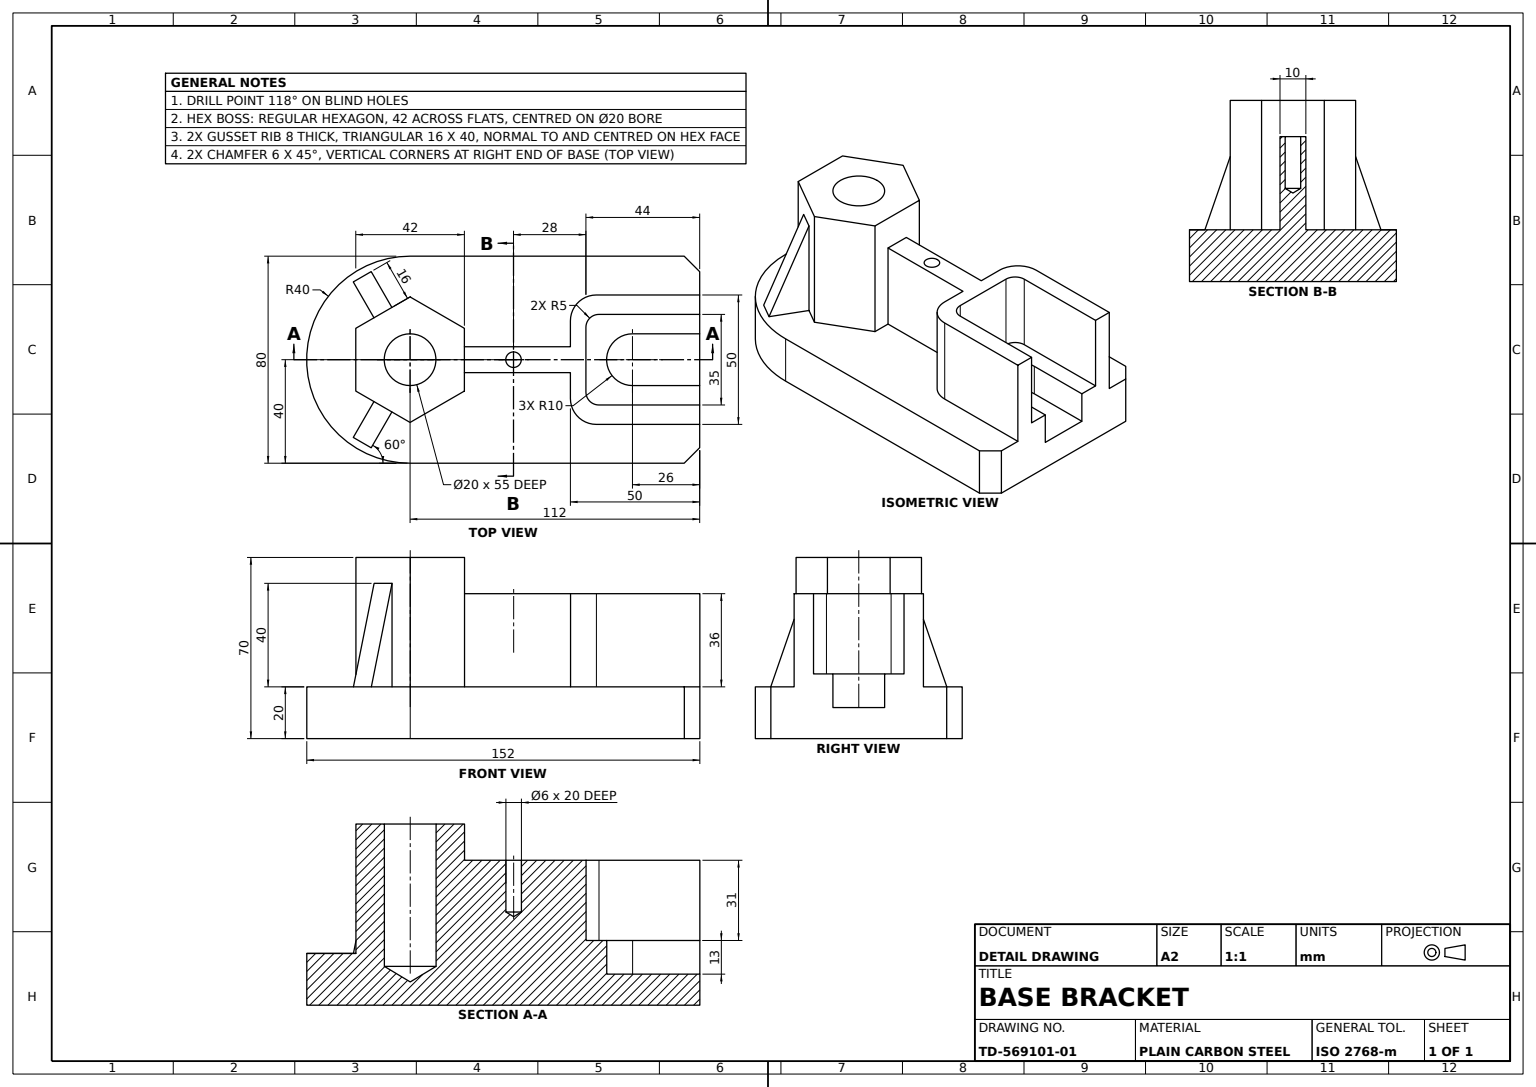
SolidWorks part; units mm, degrees
material "Plain Carbon Steel"
ref_plane "Front Plane" through (0, 0, 0) normal (0, 0, 1) x (1, 0, 0)
ref_plane "Top Plane" through (0, 0, 0) normal (0, 1, 0) x (1, 0, 0)
ref_plane "Right Plane" through (0, 0, 0) normal (1, 0, 0) x (0, 0, -1)
sketch "Base Plate Sketch" plane through (0, 0, 0) normal (0, 1, 0) x (1, 0, 0)
  line L0 (0, 40) -> (106, 40)
  line L1 (112, 34) -> (112, -34)
  line L2 (106, -40) -> (0, -40)
  line L3 (106, 40) -> (112, 34)
  line L4 (112, -34) -> (106, -40)
  arc A0 (0, 40) -> (0, -40) centre (0, 0) ccw
  point P4 (112, 40)
  point P5 (112, -40)
  dimension "D1" = 80
  dimension "D2" = 112
  dimension "D3" = 6
  dimension "D4" = 45
  dimension "D5" = 6
  dimension "D6" = 45
extrude "Base Plate" add sketch "Base Plate Sketch" along normal blind 20
sketch "Hex Boss Sketch" plane through (0, 20, 0) normal (0, 1, 0) x (1, 0, 0)
  line L1 (0, 24.2487) -> (-21, 12.1244)
  line L2 (-21, 12.1244) -> (-21, -12.1244)
  line L3 (-21, -12.1244) -> (0, -24.2487)
  line L4 (0, -24.2487) -> (21, -12.1244)
  line L5 (21, -12.1244) -> (21, 12.1244)
  line L6 (21, 12.1244) -> (0, 24.2487)
  circle A0 centre (0, 0) radius 21 construction
  dimension "D1" = 42
extrude "Hex Mounting Boss" add sketch "Hex Boss Sketch" along normal blind 50
sketch "Gusset Rib 1 Sketch" plane through (-10.5, 0, 18.1865) normal (-0.5, 0, 0.866) x (0.866, 0, 0.5)
  line L0 (-12.1244, 20) -> (12.1244, 20) construction
  line L1 (-4, 60) -> (4, 60)
  line L2 (-4, 60) -> (-4, 20)
  line L3 (-4, 20) -> (4, 20)
  line L4 (4, 60) -> (4, 20)
  line L5 (-12.1244, 70) -> (12.1244, 70) construction
  point P8 (0, 70)
  dimension "D1" = 4
  dimension "D2" = 8
  dimension "D3" = 40
extrude "Gusset Rib 1" add sketch "Gusset Rib 1 Sketch" along normal blind 16
sketch "Rib 1 Trim Sketch" plane through (3.4641, 0, 2) normal (0.866, 0, 0.5) x (0.5, 0, -0.866)
  line L0 (-21, 60) -> (-37, 20)
  line L1 (-21, 60) -> (-37, 60)
  line L2 (-37, 60) -> (-37, 20)
extrude "Rib 1 Trim Cut" cut sketch "Rib 1 Trim Sketch" against normal blind 16
sketch "Gusset Rib 2 Sketch" plane through (-10.5, 0, -18.1865) normal (-0.5, 0, -0.866) x (-0.866, 0, 0.5)
  line L0 (-12.1244, 20) -> (12.1244, 20) construction
  line L1 (-4, 60) -> (4, 60)
  line L2 (-4, 60) -> (-4, 20)
  line L3 (-4, 20) -> (4, 20)
  line L4 (4, 60) -> (4, 20)
  line L5 (-12.1244, 70) -> (12.1244, 70) construction
  point P8 (0, 70)
  dimension "D1" = 4
  dimension "D2" = 8
  dimension "D3" = 40
extrude "Gusset Rib 2" add sketch "Gusset Rib 2 Sketch" along normal blind 16
sketch "Rib 2 Trim Sketch" plane through (-3.4641, 0, 2) normal (-0.866, 0, 0.5) x (0.5, 0, 0.866)
  line L0 (-21, 60) -> (-37, 20)
  line L1 (-37, 20) -> (-37, 60)
  line L2 (-37, 60) -> (-21, 60)
extrude "Rib 2 Trim Cut" cut sketch "Rib 2 Trim Sketch" against normal blind 16
hole_wizard "Boss Bore Ø20" positions "Sketch16" profile "Sketch17" hole size "Ø20.0" standard "ISO"
sketch "Sketch16" plane through (0, 70, 0) normal (0, 1, 0) x (1, 0, 0)
  point P0 (0, 0)
sketch "Sketch17" plane through (0, 70, 0) normal (1, 0, 0) x (0, 0, 1)
  line L0 (0, 0) -> (0, 61.0086)
  line L1 (0, 61.0086) -> (10, 55)
  line L2 (10, 55) -> (10, 0)
  line L5 (10, 0) -> (0, 0)
  line L10 (0, 61.0086) -> (-10, 55) construction
  line L11 (0, -6.35) -> (0, 107.95) construction
  dimension "Hole Dia." = 20
  dimension "Hole Depth" = 55
  dimension "Drill Angle" = 118
sketch "Shaft Housing Sketch" plane through (0, 20, 0) normal (0, 1, 0) x (1, 0, 0)
  line L0 (112, -34) -> (112, 34) construction
  line L1 (112, 25) -> (62, 25)
  line L2 (112, 25) -> (112, -25)
  line L3 (112, -25) -> (62, -25)
  line L4 (62, 25) -> (62, 5)
  line L5 (21, -12.1244) -> (21, 12.1244) construction
  line L6 (21, 5) -> (62, 5)
  line L7 (21, 5) -> (21, -5)
  line L8 (21, -5) -> (62, -5)
  line L10 (62, -5) -> (62, -25)
  dimension "D1" = 25
  dimension "D2" = 50
  dimension "D3" = 50
  dimension "D4" = 5
  dimension "D5" = 10
extrude "Shaft Housing" add sketch "Shaft Housing Sketch" along normal blind 36
fillet "Housing Fillet R10" radius 10 2 edges at (62, 38, -25) (62, 38, 25)
sketch "Housing Pocket Sketch" plane through (0, 56, 0) normal (0, 1, 0) x (1, 0, 0)
  line L0 (112, -25) -> (112, 25) construction
  line L1 (112, 17.5) -> (73, 17.5)
  line L2 (112, 17.5) -> (112, -17.5)
  line L3 (112, -17.5) -> (73, -17.5)
  line L4 (68, 12.5) -> (68, -12.5)
  arc A0 (68, -12.5) -> (73, -17.5) centre (73, -12.5) ccw
  arc A1 (68, 12.5) -> (73, 17.5) centre (73, 12.5) cw
  point P11 (68, 17.5)
  dimension "D4" = 5
  dimension "D1" = 17.5
  dimension "D2" = 35
  dimension "D3" = 44
extrude "Housing Pocket" cut sketch "Housing Pocket Sketch" against normal blind 31
sketch "Housing Slot Sketch" plane through (0, 25, 0) normal (0, 1, 0) x (1, 0, 0)
  line L0 (112, -17.5) -> (112, 17.5) construction
  line L1 (86, 10) -> (112, 10)
  line L2 (112, 10) -> (112, -10)
  line L3 (112, -10) -> (86, -10)
  arc A0 (86, 10) -> (86, -10) centre (86, 0) ccw
  dimension "D1" = 20
  dimension "D2" = 26
  dimension "D3" = 10
extrude "Housing Slot" cut sketch "Housing Slot Sketch" against normal blind 13
sketch "Cross Hole Position Sketch" plane through (0, 56, 0) normal (0, 1, 0) x (1, 0, 0)
  line L0 (112, 0) -> (40, 0)
  line L1 (112, -10) -> (112, 10) construction
  line L2 (68, 12.5) -> (68, -12.5) construction
  dimension "D1" = 28
hole_wizard "Cross Hole Ø6" positions "Sketch23" profile "Sketch24" hole size "Ø6.0" standard "ISO"
sketch "Sketch23" plane through (0, 56, 0) normal (0, 1, 0) x (1, 0, 0)
  point P0 (40, 0)
sketch "Sketch24" plane through (40, 56, 0) normal (1, 0, 0) x (0, 0, 1)
  line L0 (0, 0) -> (0, 21.8026)
  line L1 (0, 21.8026) -> (3, 20)
  line L2 (3, 20) -> (3, 0)
  line L5 (3, 0) -> (0, 0)
  line L10 (0, 21.8026) -> (-3, 20) construction
  line L11 (0, -6.35) -> (0, 107.95) construction
  dimension "Hole Dia." = 6
  dimension "Hole Depth" = 20
  dimension "Drill Angle" = 118
